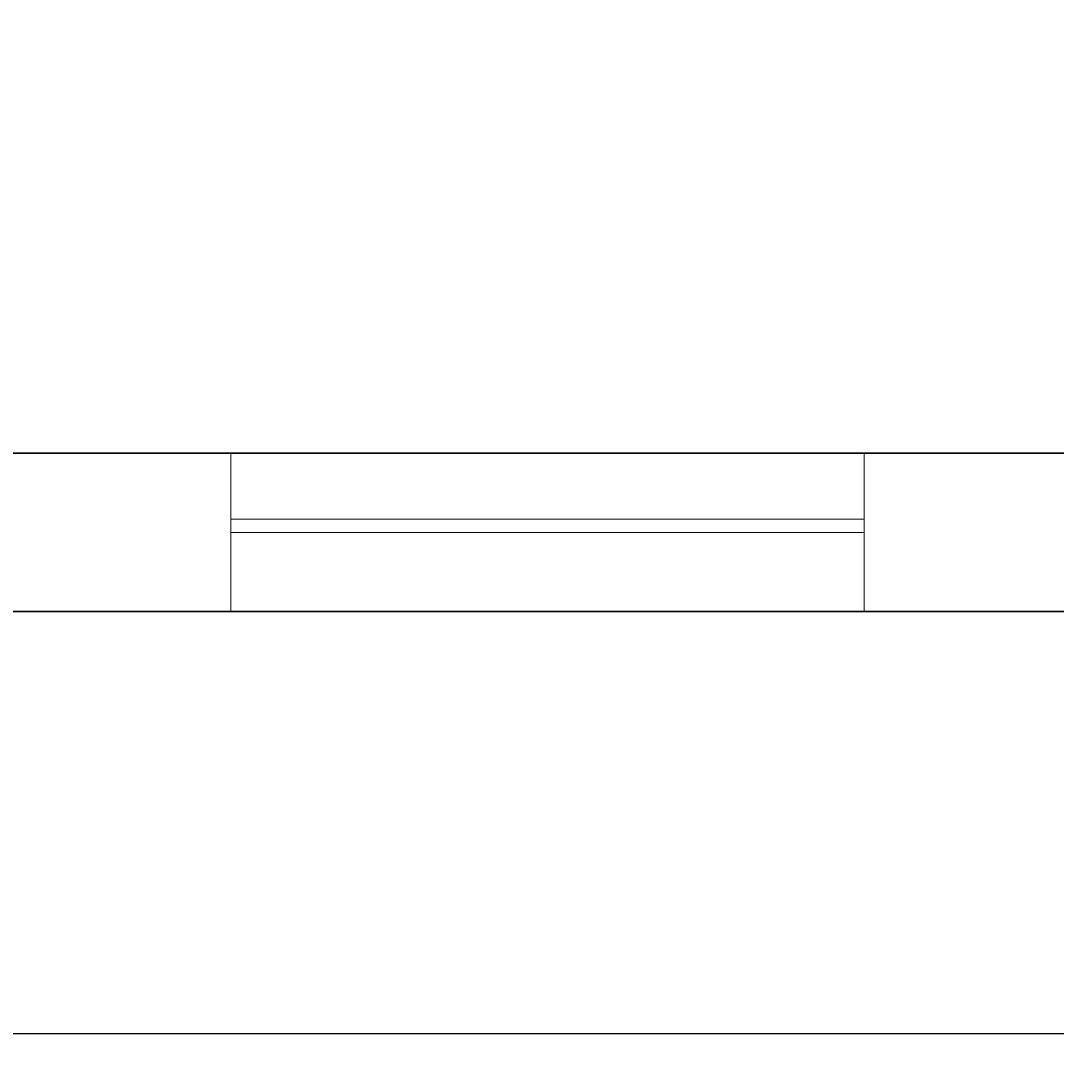
# Model space of a CAD drawing. Units: inches. Extents: x -61 to 1599, y -1316 to 257.
# Tile 10 of 204: x 200 to 259, y -1242 to -1182. Entities that reach past the tile are written whole.
import ezdxf

# ---------------------------------------------------------------- set-up
doc = ezdxf.new("R2010")
doc.units = ezdxf.units.IN
doc.header["$MEASUREMENT"] = 0
for name, color, linetype, lineweight in [('A-ANNO-DIMS', 2, 'Continuous', 18), ('WALLS', 4, 'Continuous', 35), ('WINDOWS', 220, 'Continuous', 18)]:
    doc.layers.add(name, color=color, linetype=linetype, lineweight=lineweight)
doc.styles.get("Standard").update_dxf_attribs({"font": 'arial.ttf'})
doc.dimstyles.get("Standard").update_dxf_attribs({"dimtxt": 0.18, "dimasz": 0.18, "dimexe": 0.18, "dimexo": 0.0625, "dimgap": 0.09, "dimtad": 0, "dimtih": 1, "dimtoh": 1, "dimdec": 0, "dimzin": 0, "dimdsep": 46, "dimlunit": 3, "dimtxsty": 'Standard', "dimcen": 0.09, "dimadec": 0, "dimazin": 0, "dimtfac": 1, "dimtdec": 0, "dimtofl": 0, "dimtmove": 0, "dimatfit": 3, "dimfxl": 1, "dimtolj": 1, "dimtzin": 0, "dimarcsym": 0})

# ---------------------------------------------------------------- blocks, each defined once
blk = doc.blocks.new('WIN-36IN-2')
for p, q in [((0, 9), (0, 0)), ((36, 9), (36, 0)), ((0, 5.262), (36, 5.262)), ((0, 4.5), (36, 4.5)), ((0, 4.5), (36, 4.5))]:
    blk.add_line(p, q)
blk = doc.blocks.new('*D687')
at = {"layer": 'A-ANNO-DIMS', "color": 0, "lineweight": -2, "transparency": 16777216}
for p, q in [((289.418, 181.677), (-61.077, 181.677)), ((-60.897, 181.497), (-60.897, -528.952)), ((-60.897, -1239.765), (-60.897, -529.316)), ((319.64, -1239.945), (-61.077, -1239.945))]:
    blk.add_line(p, q, dxfattribs=at)
at = {"layer": 'A-ANNO-DIMS', "color": 0, "transparency": 16777216}
for points in [[(-60.927, 181.497), (-60.867, 181.497), (-60.897, 181.677)], [(-60.927, -1239.765), (-60.867, -1239.765), (-60.897, -1239.945)]]:
    blk.add_solid(points, dxfattribs=at)
at = {"layer": 'DEFPOINTS', "color": 0, "transparency": 16777216}
for p in [(289.481, 181.677), (-60.897, -1239.945), (319.703, -1239.945)]:
    blk.add_point(p, dxfattribs=at)
at = {"layer": 'A-ANNO-DIMS', "color": 0, "transparency": 16777216, "insert": (-60.897, -529.134), "char_height": 0.18, "attachment_point": 5}
blk.add_mtext('\\A1;1421.6', dxfattribs=at)
blk = doc.blocks.new('*D688')
at = {"layer": 'A-ANNO-DIMS', "color": 0, "lineweight": -2, "transparency": 16777216}
for p, q in [((14.703, -1216.007), (14.703, -1315.725)), ((544.703, -1216.007), (544.703, -1315.725)), ((14.883, -1315.545), (279.414, -1315.545)), ((544.523, -1315.545), (279.991, -1315.545))]:
    blk.add_line(p, q, dxfattribs=at)
at = {"layer": 'A-ANNO-DIMS', "color": 0, "transparency": 16777216}
for points in [[(14.883, -1315.515), (14.883, -1315.575), (14.703, -1315.545)], [(544.523, -1315.515), (544.523, -1315.575), (544.703, -1315.545)]]:
    blk.add_solid(points, dxfattribs=at)
at = {"layer": 'DEFPOINTS', "color": 0, "transparency": 16777216}
for p in [(14.703, -1215.945), (544.703, -1215.945), (544.703, -1315.545)]:
    blk.add_point(p, dxfattribs=at)
at = {"layer": 'A-ANNO-DIMS', "color": 0, "transparency": 16777216, "insert": (279.703, -1315.545), "char_height": 0.18, "attachment_point": 5}
blk.add_mtext('\\A1;530', dxfattribs=at)

msp = doc.modelspace()

# ---------------------------------------------------------------- linework, layer by layer
at = {"layer": 'WALLS'}
for p, q in [((14.7028, -1206.9446), (237.7028, -1206.9446)), ((237.7028, -1206.9446), (327.7028, -1206.9446)), ((14.7028, -1215.9446), (237.7028, -1215.9446)), ((237.7028, -1215.9446), (327.7028, -1215.9446))]:
    msp.add_line(p, q, dxfattribs=at)

# ---------------------------------------------------------------- block references
at = {"layer": 'WINDOWS'}
msp.add_blockref('WIN-36IN-2', (212.158, -1215.9447), dxfattribs=at)

# ---------------------------------------------------------------- dimensions: what is measured, and where the dimension line sits
at = {"layer": 'A-ANNO-DIMS'}
dim = msp.add_linear_dim(base=(-60.8972, -1239.9446), p1=(289.4807, 181.6771), p2=(319.7028, -1239.9446), angle=90, dimstyle='Standard', override={"dimdec": 1, "dimlfac": 1, "dimrnd": 0, "dimzin": 0, "dimdsep": 46, "dimlunit": 2}, dxfattribs=at)
dim.commit()
dim.dimension.update_dxf_attribs({"geometry": '*D687', "text_midpoint": (-60.8972, -529.1337)})
dim = msp.add_linear_dim(base=(544.7028, -1315.5446), p1=(14.7028, -1215.9446), p2=(544.7028, -1215.9446), dimstyle='Standard', override={"dimdec": 0, "dimlfac": 1, "dimrnd": 0, "dimzin": 0, "dimdsep": 46, "dimlunit": 2}, dxfattribs=at)
dim.commit()
dim.dimension.update_dxf_attribs({"geometry": '*D688', "text_midpoint": (279.7028, -1315.5446)})

doc.saveas('drawing.dxf')
